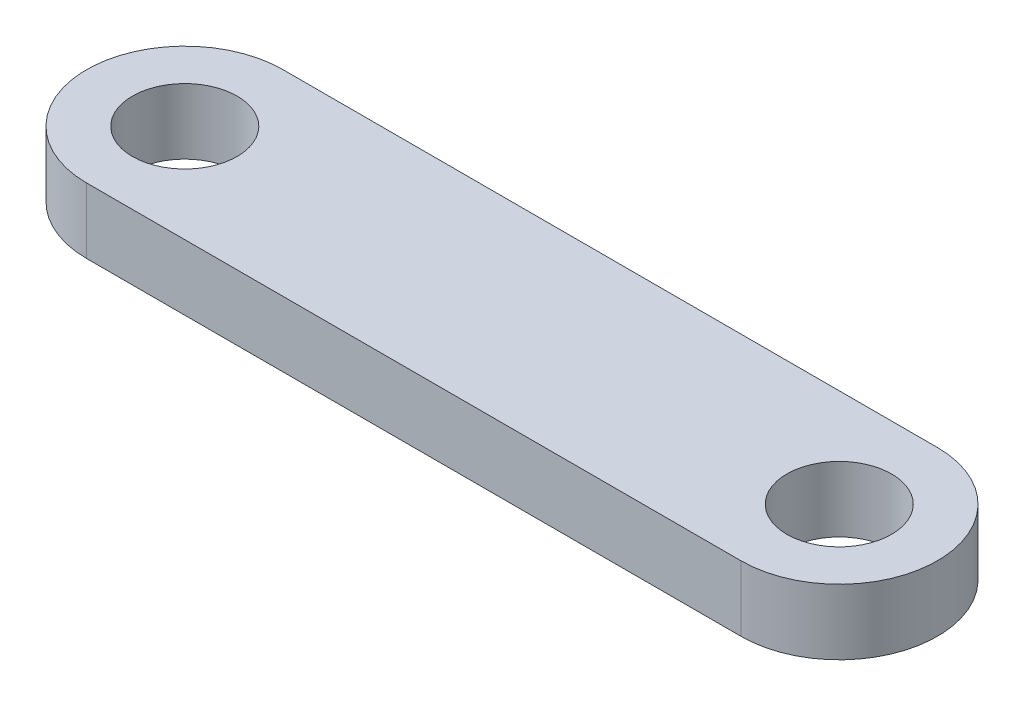
SolidWorks part; units mm, degrees
material "Plain Carbon Steel"
ref_plane "Front Plane" through (0, 0, 0) normal (0, 0, 1) x (1, 0, 0)
ref_plane "Top Plane" through (0, 0, 0) normal (0, 1, 0) x (1, 0, 0)
ref_plane "Right Plane" through (0, 0, 0) normal (1, 0, 0) x (0, 0, -1)
sketch "Link Profile Sketch" plane through (0, 0, 0) normal (0, 1, 0) x (1, 0, 0)
  line L0 (-333.1357, 0) -> (16323.6511, 0) construction
  line L1 (0, -333.1357) -> (0, 16323.6511) construction
  line L2 (-25, 0) -> (25, 0) construction
  line L3 (-25, 7.5) -> (25, 7.5)
  line L4 (-25, -7.5) -> (25, -7.5)
  arc A0 (-25, 7.5) -> (-25, -7.5) centre (-25, 0) ccw
  arc A1 (25, -7.5) -> (25, 7.5) centre (25, 0) ccw
  point P7 (0, 0)
  dimension "D1" = 7.5
  dimension "D2" = 50
  dimension "D3" = 25
extrude "Link Plate" add sketch "Link Profile Sketch" along normal mid plane 5
sketch "Pin Holes Sketch" plane through (0, 0, 0) normal (0, 1, 0) x (1, 0, 0)
  circle A0 centre (-25, 0) radius 4
  circle A1 centre (25, 0) radius 4
  dimension "D1" = 8
  dimension "D2" = 8
extrude "Pin Holes 2xØ8" cut sketch "Pin Holes Sketch" against normal mid plane 5
